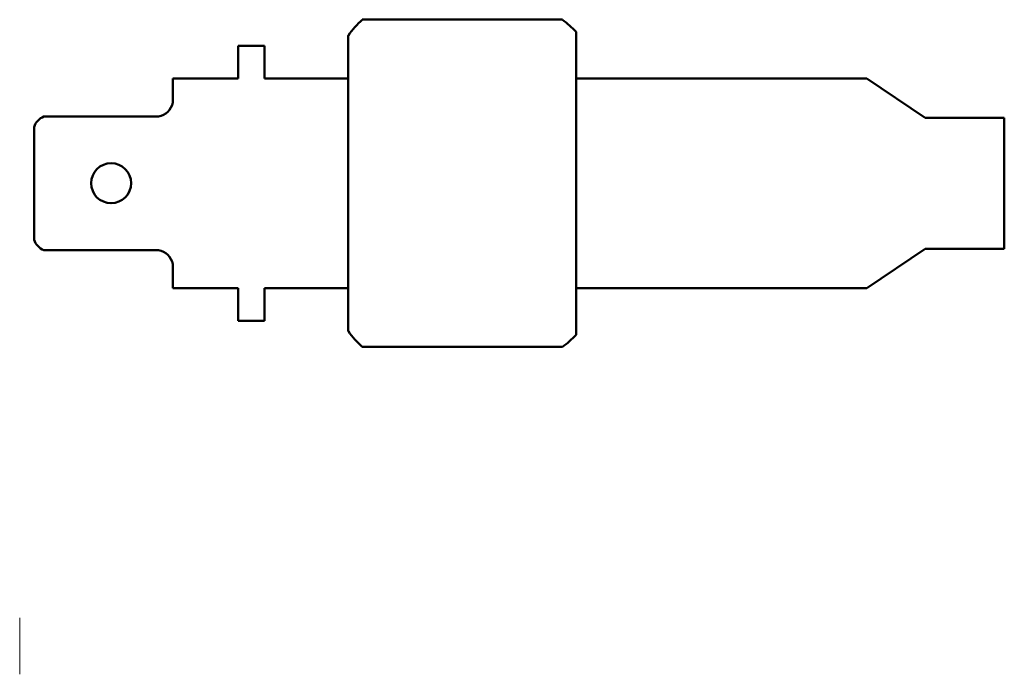
# Model space of a CAD drawing. Units: millimetres. Extents: x 1361 to 2715, y 1249 to 2149.
import ezdxf

# ---------------------------------------------------------------- set-up
doc = ezdxf.new("R2010")
doc.units = ezdxf.units.MM
doc.layers.add('M-CONS', color=8, linetype='Continuous', lineweight=13)
doc.layers.add('M-OUTL', color=7, linetype='Continuous', lineweight=50)

msp = doc.modelspace()

# ---------------------------------------------------------------- linework, layer by layer
at = {"layer": 'M-CONS'}
msp.add_line((1360.6, 1249.1), (1360.6, 1326.6), dxfattribs=at)
at = {"layer": 'M-OUTL'}
for p, q in [((1831.9, 2149.4), (2107.2, 2149.4)), ((1831.9, 2149.4), (2107.2, 2149.4)), ((1812.7, 2068.3), (1812.7, 2127.8)), ((1812.7, 2068.3), (1812.7, 2127.8)), ((2126.1, 2132.7), (2126.1, 2068.3)), ((2126.1, 2132.7), (2126.1, 2068.3)), ((1661.4, 2068.3), (1661.4, 2113.3)), ((1661.4, 2113.3), (1697.4, 2113.3)), ((1661.4, 2068.3), (1661.4, 2113.3)), ((1661.4, 2113.3), (1697.4, 2113.3)), ((1697.4, 2113.3), (1697.4, 2068.3)), ((1697.4, 2113.3), (1697.4, 2068.3)), ((1571.3, 2035.6), (1571.3, 2068.3)), ((1661.4, 2068.3), (1571.3, 2068.3)), ((1571.3, 2035.6), (1571.3, 2068.3)), ((1661.4, 2068.3), (1571.3, 2068.3)), ((1697.4, 2068.3), (1812.7, 2068.3)), ((1697.4, 2068.3), (1812.7, 2068.3)), ((1812.7, 1780.3), (1812.7, 2068.3)), ((2126.1, 2068.3), (2526, 2068.3)), ((2126.1, 2068.3), (2526, 2068.3)), ((2126.1, 1780.3), (2126.1, 2068.3)), ((2526, 2068.3), (2606.4, 2014.3)), ((2526, 2068.3), (2606.4, 2014.3)), ((1393.6, 2016.1), (1551.5, 2016.1)), ((1393.6, 2016.1), (1551.5, 2016.1)), ((2606.4, 2014.3), (2715.1, 2014.3)), ((2606.4, 2014.3), (2715.1, 2014.3)), ((2715.1, 2014.3), (2715.1, 1924.3)), ((2715.1, 2014.3), (2715.1, 1924.3)), ((1380.4, 1924.3), (1380.4, 2001.8)), ((1380.4, 1924.3), (1380.4, 2001.8)), ((1380.4, 1924.3), (1380.4, 1846.8)), ((1380.4, 1924.3), (1380.4, 1846.8)), ((2715.1, 1834.3), (2715.1, 1924.3)), ((2715.1, 1834.3), (2715.1, 1924.3)), ((1393.6, 1832.5), (1551.5, 1832.5)), ((1393.6, 1832.5), (1551.5, 1832.5)), ((2526, 1780.3), (2606.4, 1834.3)), ((2526, 1780.3), (2606.4, 1834.3)), ((2606.4, 1834.3), (2715.1, 1834.3)), ((2606.4, 1834.3), (2715.1, 1834.3)), ((1571.3, 1813), (1571.3, 1780.3)), ((1571.3, 1813), (1571.3, 1780.3)), ((1661.4, 1780.3), (1571.3, 1780.3)), ((1661.4, 1780.3), (1571.3, 1780.3)), ((1661.4, 1780.3), (1661.4, 1735.3)), ((1661.4, 1780.3), (1661.4, 1735.3)), ((1697.4, 1735.3), (1697.4, 1780.3)), ((1697.4, 1780.3), (1812.7, 1780.3)), ((1697.4, 1735.3), (1697.4, 1780.3)), ((1697.4, 1780.3), (1812.7, 1780.3)), ((1812.7, 1780.3), (1812.7, 1720.8)), ((1812.7, 1780.3), (1812.7, 1720.8)), ((2126.1, 1715.9), (2126.1, 1780.3)), ((2126.1, 1780.3), (2526, 1780.3)), ((2126.1, 1715.9), (2126.1, 1780.3)), ((2126.1, 1780.3), (2526, 1780.3)), ((1661.4, 1735.3), (1697.4, 1735.3)), ((1661.4, 1735.3), (1697.4, 1735.3)), ((1831.9, 1699.3), (2107.2, 1699.3)), ((1831.9, 1699.3), (2107.2, 1699.3))]:
    msp.add_line(p, q, dxfattribs=at)
msp.add_circle((1486.4, 1924.5), 27.5, dxfattribs=at)
for centre, radius, start, end in [((1921.8, 2049.8), 134.1, 132.0602, 144.4283), ((1921.8, 2049.8), 134.1, 132.0602, 144.4283), ((2015.1, 2025.6), 154.2, 43.9705, 53.3345), ((2015.1, 2025.6), 154.2, 43.9705, 53.3345), ((1546.7, 2040.8), 25.2, 280.8899, 348.0204), ((1546.7, 2040.8), 25.2, 280.8899, 348.0204), ((1402.2, 1995), 22.8, 112.0367, 162.7011), ((1402.2, 1995), 22.8, 112.0367, 162.7011), ((1402.2, 1853.6), 22.8, 197.2989, 247.9633), ((1402.2, 1853.6), 22.8, 197.2989, 247.9633), ((1546.7, 1807.8), 25.2, 11.9796, 79.1101), ((1546.7, 1807.8), 25.2, 11.9796, 79.1101), ((1921.8, 1798.9), 134.1, 215.5717, 227.9398), ((1921.8, 1798.9), 134.1, 215.5717, 227.9398), ((2015.1, 1823), 154.2, 306.6655, 316.0295), ((2015.1, 1823), 154.2, 306.6655, 316.0295)]:
    msp.add_arc(centre, radius, start, end, dxfattribs=at)

doc.saveas('drawing.dxf')
